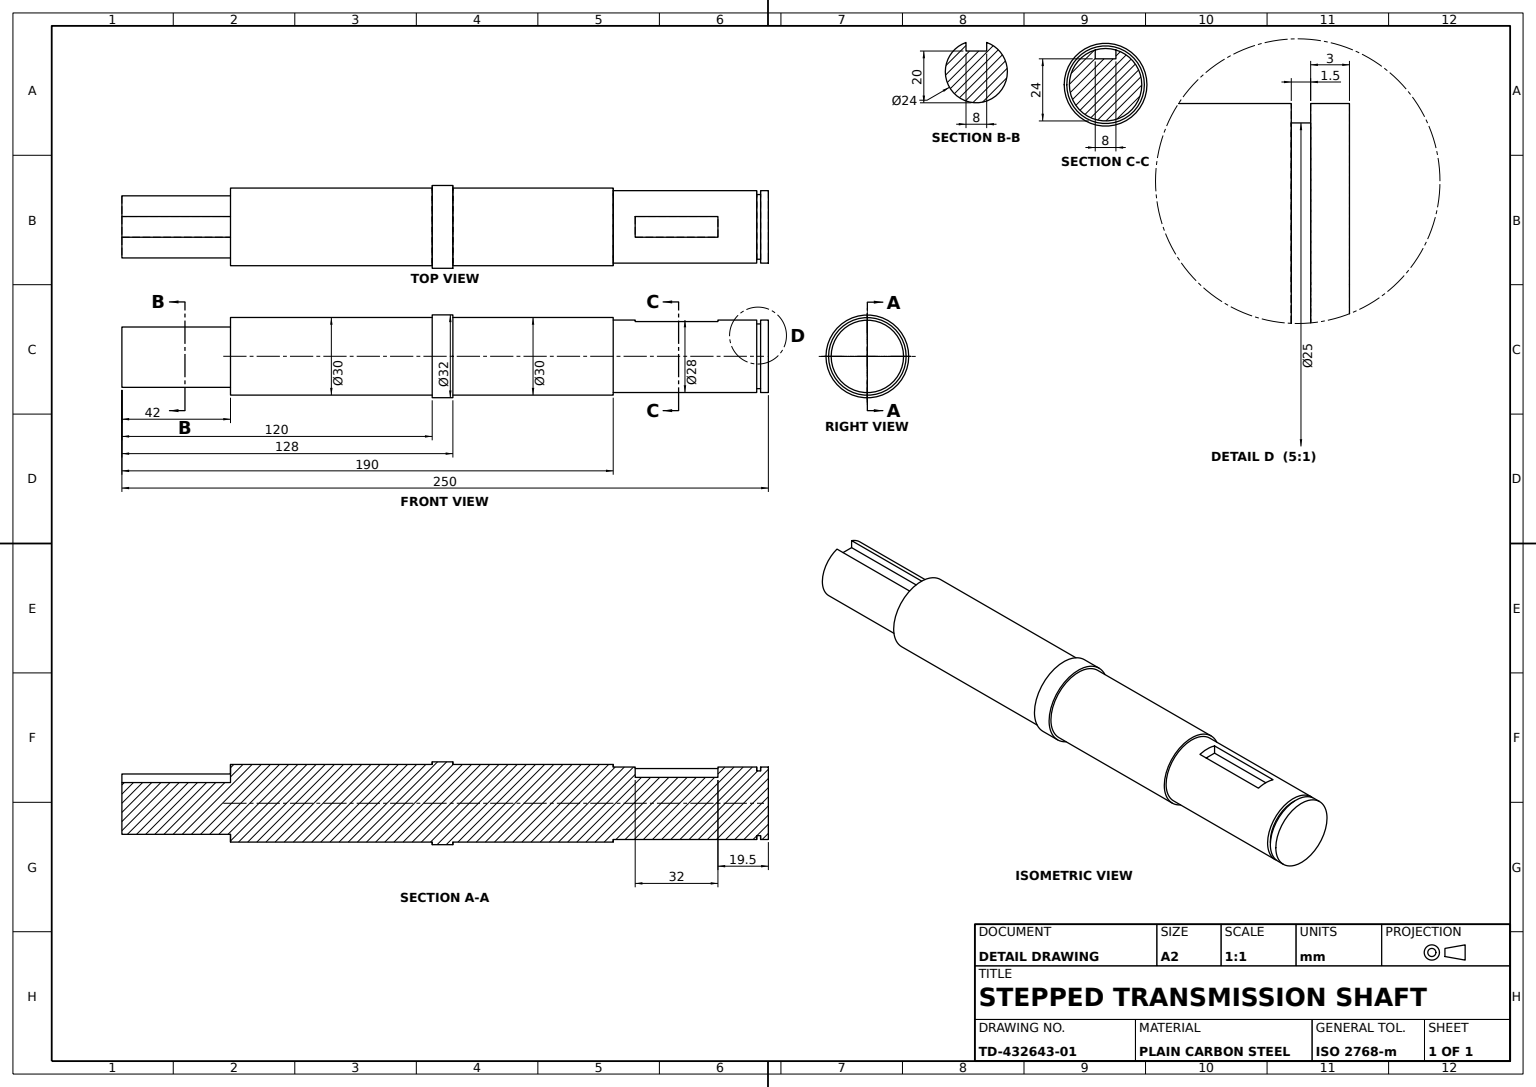
SolidWorks part; units mm, degrees
material "Plain Carbon Steel"
ref_plane "Front Plane" through (0, 0, 0) normal (0, 0, 1) x (1, 0, 0)
ref_plane "Top Plane" through (0, 0, 0) normal (0, 1, 0) x (1, 0, 0)
ref_plane "Right Plane" through (0, 0, 0) normal (1, 0, 0) x (0, 0, -1)
sketch "Shaft Profile Sketch" plane through (0, 0, 0) normal (0, 0, 1) x (1, 0, 0)
  line L0 (0, 0) -> (250, 0) construction
  line L1 (0, 0) -> (0, 12)
  line L2 (0, 12) -> (42, 12)
  line L3 (42, 12) -> (42, 15)
  line L4 (42, 15) -> (120, 15)
  line L5 (120, 15) -> (120, 16)
  line L6 (120, 16) -> (128, 16)
  line L7 (128, 16) -> (128, 15)
  line L8 (128, 15) -> (190, 15)
  line L9 (190, 15) -> (190, 14)
  line L10 (190, 14) -> (245.5, 14)
  line L11 (245.5, 14) -> (245.5, 12.5)
  line L12 (245.5, 12.5) -> (247, 12.5)
  line L13 (247, 12.5) -> (247, 14)
  line L14 (247, 14) -> (250, 14)
  line L15 (250, 14) -> (250, 0)
  line L16 (0, 0) -> (250, 0)
  dimension "D1" = 250
  dimension "D2" = 12
  dimension "D3" = 42
  dimension "D4" = 15
  dimension "D5" = 120
  dimension "D6" = 16
  dimension "D7" = 128
  dimension "D8" = 15
  dimension "D9" = 190
  dimension "D10" = 14
  dimension "D11" = 3
  dimension "D12" = 1.5
  dimension "D13" = 1.5
  dimension "D14" = 14
  dimension "D15" = 1
revolve "Stepped Shaft Body" add sketch "Shaft Profile Sketch" angle 360 about L0
ref_plane "Keyway 1 Plane" through (0, 12, 0) normal (0, 1, 0) x (1, 0, 0)
sketch "Keyway 1 Sketch" plane through (0, 12, 0) normal (0, 1, 0) x (1, 0, 0)
  line L0 (0, 12) -> (0, -12) construction
  line L1 (0, 4) -> (42, 4)
  line L2 (0, 4) -> (0, -4)
  line L3 (0, -4) -> (42, -4)
  line L4 (42, 4) -> (42, -4)
  line L5 (42, 12) -> (42, -12) construction
  dimension "D1" = 8
  dimension "D2" = 4
extrude "Keyway 1 Cut" cut sketch "Keyway 1 Sketch" against normal blind 4
ref_plane "Keyway 2 Plane" through (0, 14, 0) normal (0, 1, 0) x (1, 0, 0)
sketch "Keyway 2 Sketch" plane through (0, 14, 0) normal (0, 1, 0) x (1, 0, 0)
  line L0 (245.5, -14) -> (245.5, 14) construction
  line L1 (198.5, 4) -> (230.5, 4)
  line L2 (198.5, 4) -> (198.5, -4)
  line L3 (198.5, -4) -> (230.5, -4)
  line L4 (230.5, 4) -> (230.5, -4)
  line L5 (245.5, 14) -> (190, 14) construction
  point P6 (230.5, 0)
  dimension "D1" = 8
  dimension "D2" = 15
  dimension "D3" = 14
  dimension "D4" = 32
extrude "Keyway 2 Cut" cut sketch "Keyway 2 Sketch" against normal blind 4
